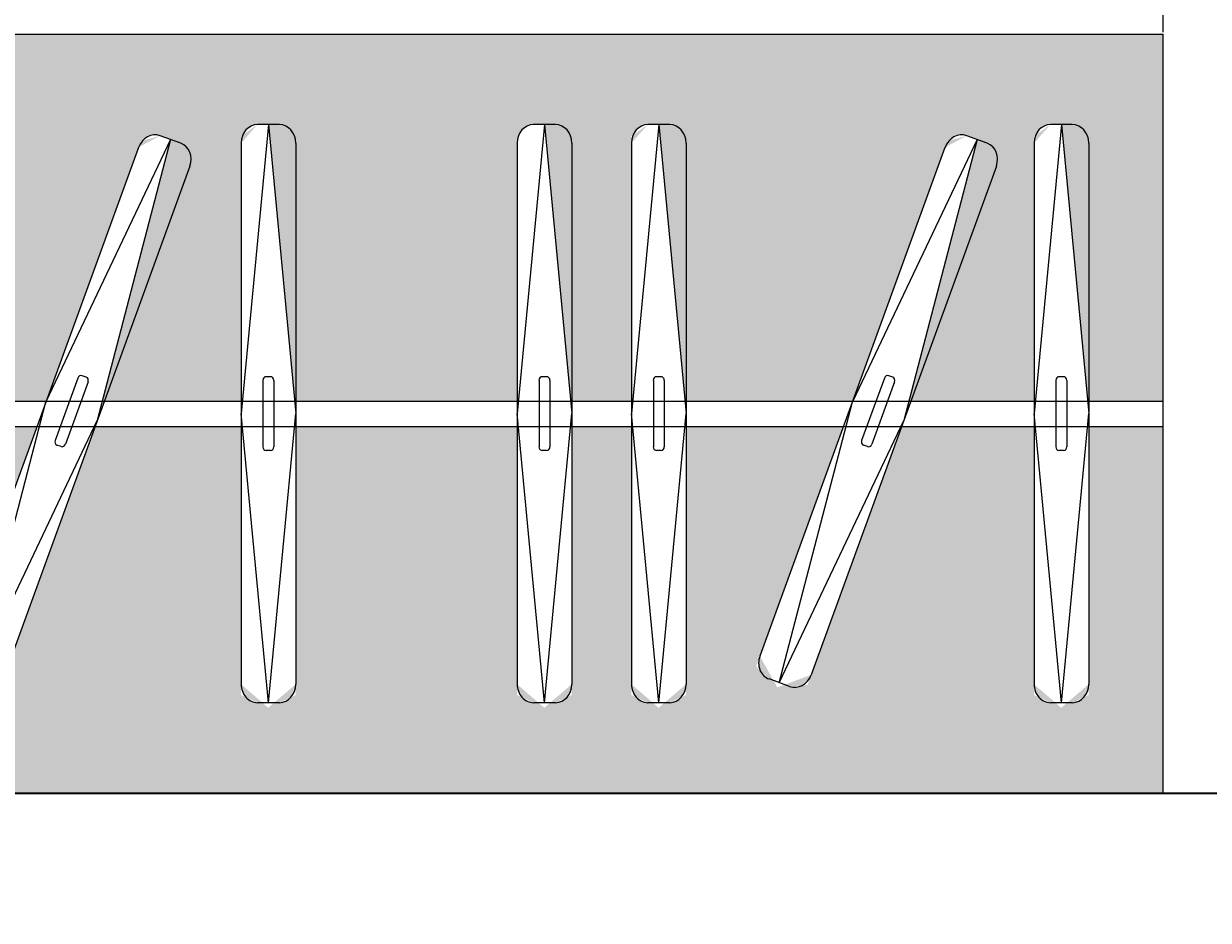
# Model space of a CAD drawing. Units: millimetres. Extents: x 27017497 to 27018854, y 7058029 to 7059154.
# Tile 40 of 91: x 27017655 to 27017689, y 7058433 to 7058459. Entities that reach past the tile are written whole.
import ezdxf

# ---------------------------------------------------------------- set-up
doc = ezdxf.new("R2010")
doc.units = ezdxf.units.MM
for name, color, linetype, lineweight in [('A-ANNO-DIMS', 2, 'Continuous', 18), ('A-FLOR-CASE', 8, 'Continuous', 20), ('A-FLOR-CASE-PATT', 44, 'Continuous', 13), ('A-WALL', 7, 'Continuous', 35)]:
    doc.layers.add(name, color=color, linetype=linetype, lineweight=lineweight)
doc.styles.get("Standard").update_dxf_attribs({"font": 'arial.ttf'})
doc.dimstyles.get("Standard").update_dxf_attribs({"dimtxt": 0.18, "dimasz": 0.18, "dimexe": 0.18, "dimexo": 0.0625, "dimgap": 0.09, "dimtad": 0, "dimtih": 1, "dimtoh": 1, "dimdec": 4, "dimzin": 0, "dimdsep": 46, "dimtxsty": 'Standard', "dimcen": 0.09, "dimadec": 0, "dimazin": 0, "dimtfac": 1, "dimtdec": 4, "dimtofl": 0, "dimtmove": 0, "dimatfit": 3, "dimfxl": 1, "dimtolj": 1, "dimtzin": 0, "dimarcsym": 0})

# ---------------------------------------------------------------- blocks, each defined once
blk = doc.blocks.new('WARDROBE-HANGING-WALL-BACKED')
for p, q in [((0, 21.737), (65.212, 21.737)), ((65.212, 0), (65.212, 21.737)), ((39.589, 19.152), (38.806, 10.877)), ((39.902, 19.152), (39.276, 19.152)), ((39.589, 19.152), (40.371, 10.877)), ((47.493, 19.152), (46.71, 10.877)), ((47.806, 19.152), (47.18, 19.152)), ((47.493, 19.152), (48.275, 10.877)), ((50.766, 19.152), (49.984, 10.877)), ((51.079, 19.152), (50.453, 19.152)), ((50.766, 19.152), (51.549, 10.877)), ((62.293, 19.152), (61.511, 10.877)), ((62.606, 19.152), (61.98, 19.152)), ((62.293, 19.152), (63.076, 10.877)), ((36.783, 18.725), (33.217, 11.217)), ((36.783, 18.725), (34.688, 10.682)), ((37.077, 18.618), (36.488, 18.833)), ((59.877, 18.725), (56.311, 11.217)), ((59.877, 18.725), (57.782, 10.682)), ((60.171, 18.618), (59.582, 18.833)), ((35.867, 18.497), (30.567, 3.937)), ((38.806, 18.624), (38.806, 3.13)), ((40.371, 18.624), (40.371, 3.13)), ((46.71, 18.624), (46.71, 3.13)), ((48.275, 18.624), (48.275, 3.13)), ((49.984, 18.624), (49.984, 3.13)), ((51.549, 18.624), (51.549, 3.13)), ((58.96, 18.497), (53.661, 3.937)), ((61.511, 18.624), (61.511, 3.13)), ((63.076, 18.624), (63.076, 3.13)), ((37.337, 17.961), (32.038, 3.402)), ((60.431, 17.961), (55.132, 3.402)), ((34.13, 11.896), (33.48, 10.109)), ((34.372, 11.92), (34.255, 11.963)), ((39.651, 11.933), (39.526, 11.933)), ((47.555, 11.933), (47.43, 11.933)), ((50.829, 11.933), (50.703, 11.933)), ((57.224, 11.896), (56.574, 10.109)), ((57.466, 11.92), (57.349, 11.963)), ((62.356, 11.933), (62.231, 11.933)), ((34.424, 11.789), (33.774, 10.002)), ((39.432, 11.828), (39.432, 9.926)), ((39.745, 11.828), (39.745, 9.926)), ((47.336, 11.828), (47.336, 9.926)), ((47.649, 11.828), (47.649, 9.926)), ((50.61, 11.828), (50.61, 9.926)), ((50.923, 11.828), (50.923, 9.926)), ((57.518, 11.789), (56.868, 10.002)), ((62.137, 11.828), (62.137, 9.926)), ((62.45, 11.828), (62.45, 9.926)), ((0, 11.231), (65.212, 11.231)), ((31.122, 3.173), (33.217, 11.217)), ((54.216, 3.173), (56.311, 11.217)), ((39.589, 2.602), (38.806, 10.877)), ((39.589, 2.602), (40.371, 10.877)), ((47.493, 2.602), (46.71, 10.877)), ((47.493, 2.602), (48.275, 10.877)), ((50.766, 2.602), (49.984, 10.877)), ((50.766, 2.602), (51.549, 10.877)), ((62.293, 2.602), (61.511, 10.877)), ((62.293, 2.602), (63.076, 10.877)), ((31.122, 3.173), (34.688, 10.682)), ((54.216, 3.173), (57.782, 10.682)), ((0, 10.506), (65.212, 10.506)), ((33.65, 9.935), (33.532, 9.978)), ((56.744, 9.935), (56.626, 9.978)), ((39.651, 9.821), (39.526, 9.821)), ((47.555, 9.821), (47.43, 9.821)), ((50.829, 9.821), (50.703, 9.821)), ((62.356, 9.821), (62.231, 9.821)), ((54.51, 3.066), (53.922, 3.28)), ((39.902, 2.602), (39.276, 2.602)), ((47.806, 2.602), (47.18, 2.602)), ((51.079, 2.602), (50.453, 2.602)), ((62.606, 2.602), (61.98, 2.602))]:
    blk.add_line(p, q)
for centre, major_axis, start_param, end_param in [((39.276, 18.624), (0, 0.528), 0, 1.570796), ((39.902, 18.624), (0, 0.528), 4.712389, 6.283185), ((47.18, 18.624), (0, 0.528), 0, 1.570796), ((47.806, 18.624), (0, 0.528), 4.712389, 6.283185), ((50.453, 18.624), (0, 0.528), 0, 1.570796), ((51.079, 18.624), (0, 0.528), 4.712389, 6.283185), ((61.98, 18.624), (0, 0.528), 0, 1.570796), ((62.606, 18.624), (0, 0.528), 4.712389, 6.283185), ((36.308, 18.336), (0.181, 0.496), 0, 1.570796), ((59.402, 18.336), (0.181, 0.496), 0, 1.570796), ((36.896, 18.122), (0.181, 0.496), -1.570796, 0), ((59.99, 18.122), (0.181, 0.496), -1.570796, 0), ((34.219, 11.864), (0.0361, 0.0993), 0, 1.570796), ((34.336, 11.821), (0.0361, 0.0993), 4.712389, 6.283185), ((39.526, 11.828), (0, 0.106), 0, 1.570796), ((39.651, 11.828), (0, 0.106), -1.570796, 0), ((47.43, 11.828), (0, 0.106), 0, 1.570796), ((47.555, 11.828), (0, 0.106), -1.570796, 0), ((50.703, 11.828), (0, 0.106), 0, 1.570796), ((50.829, 11.828), (0, 0.106), -1.570796, 0), ((57.313, 11.864), (0.0361, 0.0993), 0, 1.570796), ((57.43, 11.821), (0.0361, 0.0993), 4.712389, 6.283185), ((62.231, 11.828), (0, 0.106), 0, 1.570796), ((62.356, 11.828), (0, 0.106), -1.570796, 0), ((33.568, 10.077), (0.0361, 0.0993), 1.570796, 3.141593), ((33.686, 10.034), (0.0361, 0.0993), 3.141593, 4.712389), ((39.526, 9.926), (0, 0.106), 1.570796, 3.141593), ((39.651, 9.926), (0, 0.106), 3.141593, 4.712389), ((47.43, 9.926), (0, 0.106), 1.570796, 3.141593), ((47.555, 9.926), (0, 0.106), 3.141593, 4.712389), ((50.703, 9.926), (0, 0.106), 1.570796, 3.141593), ((50.829, 9.926), (0, 0.106), 3.141593, 4.712389), ((56.662, 10.077), (0.0361, 0.0993), 1.570796, 3.141593), ((56.78, 10.034), (0.0361, 0.0993), 3.141593, 4.712389), ((62.231, 9.926), (0, 0.106), 1.570796, 3.141593), ((62.356, 9.926), (0, 0.106), 3.141593, 4.712389), ((54.102, 3.776), (0.181, 0.496), 1.570796, 3.141593), ((54.691, 3.562), (0.181, 0.496), 3.141593, 4.712389), ((39.276, 3.13), (0, 0.528), 1.570796, 3.141593), ((39.902, 3.13), (0, 0.528), 3.141593, 4.712389), ((47.18, 3.13), (0, 0.528), 1.570796, 3.141593), ((47.806, 3.13), (0, 0.528), 3.141593, 4.712389), ((50.453, 3.13), (0, 0.528), 1.570796, 3.141593), ((51.079, 3.13), (0, 0.528), 3.141593, 4.712389), ((61.98, 3.13), (0, 0.528), 1.570796, 3.141593), ((62.606, 3.13), (0, 0.528), 3.141593, 4.712389)]:
    blk.add_ellipse(centre, major_axis=major_axis, ratio=0.888892, start_param=start_param, end_param=end_param)
blk = doc.blocks.new('*D45')
at = {"layer": 'A-ANNO-DIMS', "color": 0, "lineweight": -2, "transparency": 16777216}
for p, q in [((27017622.665, 7058458.704), (27017622.665, 7058468.604)), ((27017687.877, 7058458.704), (27017687.877, 7058468.604)), ((27017622.845, 7058468.424), (27017653.586, 7058468.424)), ((27017687.697, 7058468.424), (27017656.955, 7058468.424))]:
    blk.add_line(p, q, dxfattribs=at)
at = {"layer": 'A-ANNO-DIMS', "color": 0, "transparency": 16777216}
for points in [[(27017622.845, 7058468.454), (27017622.845, 7058468.394), (27017622.665, 7058468.424)], [(27017687.697, 7058468.454), (27017687.697, 7058468.394), (27017687.877, 7058468.424)]]:
    blk.add_solid(points, dxfattribs=at)
at = {"layer": 'Defpoints', "color": 0, "transparency": 16777216}
for p in [(27017687.877, 7058468.424), (27017622.665, 7058458.642), (27017687.877, 7058458.642)]:
    blk.add_point(p, dxfattribs=at)
at = {"layer": 'A-ANNO-DIMS', "color": 0, "transparency": 16777216, "insert": (27017655.271, 7058468.424), "char_height": 0.18, "attachment_point": 5}
blk.add_mtext('\\A1;WALL WARDROBE 65 TYP.', dxfattribs=at)
blk = doc.blocks.new('*D48')
at = {"layer": 'A-ANNO-DIMS', "color": 0, "lineweight": -2, "transparency": 16777216}
for p, q in [((27018463.498, 7058622.912), (27017497.536, 7058622.912)), ((27017497.716, 7058622.732), (27017497.716, 7058357.753)), ((27017497.716, 7058092.41), (27017497.716, 7058357.389)), ((27018555.129, 7058092.23), (27017497.536, 7058092.23))]:
    blk.add_line(p, q, dxfattribs=at)
at = {"layer": 'A-ANNO-DIMS', "color": 0, "transparency": 16777216}
for points in [[(27017497.686, 7058622.732), (27017497.746, 7058622.732), (27017497.716, 7058622.912)], [(27017497.686, 7058092.41), (27017497.746, 7058092.41), (27017497.716, 7058092.23)]]:
    blk.add_solid(points, dxfattribs=at)
at = {"layer": 'Defpoints', "color": 0, "transparency": 16777216}
for p in [(27018463.561, 7058622.912), (27017497.716, 7058092.23), (27018555.192, 7058092.23)]:
    blk.add_point(p, dxfattribs=at)
at = {"layer": 'A-ANNO-DIMS', "color": 0, "transparency": 16777216, "insert": (27017497.716, 7058357.571), "char_height": 0.18, "attachment_point": 5}
blk.add_mtext('\\A1;530.7', dxfattribs=at)

msp = doc.modelspace()

# ---------------------------------------------------------------- hatches: boundary and pattern name
at = {"layer": 'A-FLOR-CASE-PATT'}
h = msp.add_hatch(color=256, dxfattribs=at)
h.dxf.hatch_style = 1
edge = h.paths.add_edge_path()
edge.add_line((27017641.545, 7058447.411), (27017637.752, 7058447.411))
edge.add_line((27017637.752, 7058447.411), (27017635.06, 7058440.016))
edge.add_ellipse((27017634.725, 7058440.467), major_axis=(0.181, 0.496), ratio=0.888892, start_angle=180, end_angle=270, ccw=False)
edge.add_line((27017634.184, 7058439.939), (27017634.19, 7058439.951))
edge.add_ellipse((27017634.137, 7058440.681), major_axis=(0.181, 0.496), ratio=0.888892, start_angle=90, end_angle=180, ccw=False)
edge.add_line((27017633.59, 7058440.551), (27017636.086, 7058447.411))
edge.add_line((27017636.086, 7058447.411), (27017631.583, 7058447.411))
edge.add_line((27017631.583, 7058447.411), (27017631.583, 7058439.726))
edge.add_ellipse((27017631.113, 7058440.035), major_axis=(0, 0.528), ratio=0.888892, start_angle=180, end_angle=270, ccw=False)
edge.add_line((27017630.786, 7058439.354), (27017630.787, 7058439.367))
edge.add_ellipse((27017630.487, 7058440.035), major_axis=(0, 0.528), ratio=0.888892, start_angle=90, end_angle=180, ccw=False)
edge.add_line((27017630.018, 7058439.726), (27017630.018, 7058447.411))
edge.add_line((27017630.018, 7058447.411), (27017628.31, 7058447.411))
edge.add_line((27017628.31, 7058447.411), (27017628.31, 7058439.726))
edge.add_ellipse((27017627.84, 7058440.035), major_axis=(0, 0.528), ratio=0.888892, start_angle=180, end_angle=270, ccw=False)
edge.add_line((27017627.513, 7058439.354), (27017627.514, 7058439.367))
edge.add_ellipse((27017627.214, 7058440.035), major_axis=(0, 0.528), ratio=0.888892, start_angle=90, end_angle=180, ccw=False)
edge.add_line((27017626.745, 7058439.726), (27017626.745, 7058447.411))
edge.add_line((27017626.745, 7058447.411), (27017622.666, 7058447.411))
edge.add_line((27017622.666, 7058447.411), (27017622.666, 7058436.912))
edge.add_line((27017622.666, 7058436.912), (27017687.877, 7058436.912))
edge.add_line((27017687.877, 7058436.912), (27017687.877, 7058447.411))
edge.add_line((27017687.877, 7058447.411), (27017685.741, 7058447.411))
edge.add_line((27017685.741, 7058447.411), (27017685.741, 7058439.726))
edge.add_ellipse((27017685.271, 7058440.035), major_axis=(0, 0.528), ratio=0.888892, start_angle=180, end_angle=270, ccw=False)
edge.add_line((27017684.944, 7058439.354), (27017684.945, 7058439.367))
edge.add_ellipse((27017684.645, 7058440.035), major_axis=(0, 0.528), ratio=0.888892, start_angle=90, end_angle=180, ccw=False)
edge.add_line((27017684.176, 7058439.726), (27017684.176, 7058447.411))
edge.add_line((27017684.176, 7058447.411), (27017680.383, 7058447.411))
edge.add_line((27017680.383, 7058447.411), (27017677.691, 7058440.016))
edge.add_ellipse((27017677.356, 7058440.467), major_axis=(0.181, 0.496), ratio=0.888892, start_angle=180, end_angle=270, ccw=False)
edge.add_line((27017676.815, 7058439.939), (27017676.821, 7058439.951))
edge.add_ellipse((27017676.767, 7058440.681), major_axis=(0.181, 0.496), ratio=0.888892, start_angle=90, end_angle=180, ccw=False)
edge.add_line((27017676.22, 7058440.551), (27017678.717, 7058447.411))
edge.add_line((27017678.717, 7058447.411), (27017674.214, 7058447.411))
edge.add_line((27017674.214, 7058447.411), (27017674.214, 7058439.726))
edge.add_ellipse((27017673.744, 7058440.035), major_axis=(0, 0.528), ratio=0.888892, start_angle=180, end_angle=270, ccw=False)
edge.add_line((27017673.417, 7058439.354), (27017673.418, 7058439.367))
edge.add_ellipse((27017673.118, 7058440.035), major_axis=(0, 0.528), ratio=0.888892, start_angle=90, end_angle=180, ccw=False)
edge.add_line((27017672.649, 7058439.726), (27017672.649, 7058447.411))
edge.add_line((27017672.649, 7058447.411), (27017670.94, 7058447.411))
edge.add_line((27017670.94, 7058447.411), (27017670.94, 7058439.726))
edge.add_ellipse((27017670.471, 7058440.035), major_axis=(0, 0.528), ratio=0.888892, start_angle=180, end_angle=270, ccw=False)
edge.add_line((27017670.143, 7058439.354), (27017670.145, 7058439.367))
edge.add_ellipse((27017669.845, 7058440.035), major_axis=(0, 0.528), ratio=0.888892, start_angle=90, end_angle=180, ccw=False)
edge.add_line((27017669.375, 7058439.726), (27017669.375, 7058447.411))
edge.add_line((27017669.375, 7058447.411), (27017663.036, 7058447.411))
edge.add_line((27017663.036, 7058447.411), (27017663.036, 7058439.726))
edge.add_ellipse((27017662.567, 7058440.035), major_axis=(0, 0.528), ratio=0.888892, start_angle=180, end_angle=270, ccw=False)
edge.add_line((27017662.239, 7058439.354), (27017662.241, 7058439.367))
edge.add_ellipse((27017661.941, 7058440.035), major_axis=(0, 0.528), ratio=0.888892, start_angle=90, end_angle=180, ccw=False)
edge.add_line((27017661.471, 7058439.726), (27017661.471, 7058447.411))
edge.add_line((27017661.471, 7058447.411), (27017657.289, 7058447.411))
edge.add_line((27017657.289, 7058447.411), (27017654.597, 7058440.016))
edge.add_ellipse((27017654.262, 7058440.467), major_axis=(0.181, 0.496), ratio=0.888892, start_angle=180, end_angle=270, ccw=False)
edge.add_line((27017653.721, 7058439.939), (27017653.727, 7058439.951))
edge.add_ellipse((27017653.673, 7058440.681), major_axis=(0.181, 0.496), ratio=0.888892, start_angle=90, end_angle=180, ccw=False)
edge.add_line((27017653.126, 7058440.551), (27017655.623, 7058447.411))
edge.add_line((27017655.623, 7058447.411), (27017652.621, 7058447.411))
edge.add_line((27017652.621, 7058447.411), (27017652.621, 7058439.726))
edge.add_ellipse((27017652.151, 7058440.035), major_axis=(0, 0.528), ratio=0.888892, start_angle=180, end_angle=270, ccw=False)
edge.add_line((27017651.824, 7058439.354), (27017651.825, 7058439.367))
edge.add_ellipse((27017651.525, 7058440.035), major_axis=(0, 0.528), ratio=0.888892, start_angle=90, end_angle=180, ccw=False)
edge.add_line((27017651.056, 7058439.726), (27017651.056, 7058447.411))
edge.add_line((27017651.056, 7058447.411), (27017649.348, 7058447.411))
edge.add_line((27017649.348, 7058447.411), (27017649.348, 7058439.726))
edge.add_ellipse((27017648.878, 7058440.035), major_axis=(0, 0.528), ratio=0.888892, start_angle=180, end_angle=270, ccw=False)
edge.add_line((27017648.551, 7058439.354), (27017648.552, 7058439.367))
edge.add_ellipse((27017648.252, 7058440.035), major_axis=(0, 0.528), ratio=0.888892, start_angle=90, end_angle=180, ccw=False)
edge.add_line((27017647.783, 7058439.726), (27017647.783, 7058447.411))
edge.add_line((27017647.783, 7058447.411), (27017643.11, 7058447.411))
edge.add_line((27017643.11, 7058447.411), (27017643.11, 7058439.726))
edge.add_ellipse((27017642.641, 7058440.035), major_axis=(0, 0.528), ratio=0.888892, start_angle=180, end_angle=270, ccw=False)
edge.add_line((27017642.313, 7058439.354), (27017642.314, 7058439.367))
edge.add_ellipse((27017642.015, 7058440.035), major_axis=(0, 0.528), ratio=0.888892, start_angle=90, end_angle=180, ccw=False)
edge.add_line((27017641.545, 7058439.726), (27017641.545, 7058447.411))
edge = h.paths.add_edge_path()
edge.add_line((27017669.845, 7058456.057), (27017670.158, 7058456.057))
edge.add_line((27017670.158, 7058456.057), (27017670.907, 7058448.136))
edge.add_line((27017670.907, 7058448.136), (27017672.649, 7058448.136))
edge.add_line((27017672.649, 7058448.136), (27017672.649, 7058455.723))
edge.add_ellipse((27017673.118, 7058455.529), major_axis=(0, 0.528), ratio=0.888892, start_angle=0, end_angle=90, ccw=False)
edge.add_line((27017673.118, 7058456.057), (27017673.431, 7058456.057))
edge.add_line((27017673.431, 7058456.057), (27017674.18, 7058448.136))
edge.add_line((27017674.18, 7058448.136), (27017678.981, 7058448.136))
edge.add_line((27017678.981, 7058448.136), (27017681.692, 7058455.583))
edge.add_ellipse((27017682.067, 7058455.241), major_axis=(0.181, 0.496), ratio=0.888892, start_angle=0, end_angle=90, ccw=False)
edge.add_line((27017682.247, 7058455.738), (27017682.542, 7058455.63))
edge.add_line((27017682.542, 7058455.63), (27017680.59, 7058448.136))
edge.add_line((27017680.59, 7058448.136), (27017684.176, 7058448.136))
edge.add_line((27017684.176, 7058448.136), (27017684.176, 7058455.723))
edge.add_ellipse((27017684.645, 7058455.529), major_axis=(0, 0.528), ratio=0.888892, start_angle=0, end_angle=90, ccw=False)
edge.add_line((27017684.645, 7058456.057), (27017684.958, 7058456.057))
edge.add_line((27017684.958, 7058456.057), (27017685.707, 7058448.136))
edge.add_line((27017685.707, 7058448.136), (27017687.877, 7058448.136))
edge.add_line((27017687.877, 7058448.136), (27017687.877, 7058458.642))
edge.add_line((27017687.877, 7058458.642), (27017622.666, 7058458.642))
edge.add_line((27017622.666, 7058458.642), (27017622.666, 7058448.136))
edge.add_line((27017622.666, 7058448.136), (27017626.745, 7058448.136))
edge.add_line((27017626.745, 7058448.136), (27017626.745, 7058455.723))
edge.add_ellipse((27017627.214, 7058455.529), major_axis=(0, 0.528), ratio=0.888892, start_angle=0, end_angle=90, ccw=False)
edge.add_line((27017627.214, 7058456.057), (27017627.527, 7058456.057))
edge.add_line((27017627.527, 7058456.057), (27017628.276, 7058448.136))
edge.add_line((27017628.276, 7058448.136), (27017630.018, 7058448.136))
edge.add_line((27017630.018, 7058448.136), (27017630.018, 7058455.723))
edge.add_ellipse((27017630.487, 7058455.529), major_axis=(0, 0.528), ratio=0.888892, start_angle=0, end_angle=90, ccw=False)
edge.add_line((27017630.487, 7058456.057), (27017630.8, 7058456.057))
edge.add_line((27017630.8, 7058456.057), (27017631.549, 7058448.136))
edge.add_line((27017631.549, 7058448.136), (27017636.35, 7058448.136))
edge.add_line((27017636.35, 7058448.136), (27017639.061, 7058455.583))
edge.add_ellipse((27017639.436, 7058455.241), major_axis=(0.181, 0.496), ratio=0.888892, start_angle=0, end_angle=90, ccw=False)
edge.add_line((27017639.617, 7058455.738), (27017639.911, 7058455.63))
edge.add_line((27017639.911, 7058455.63), (27017637.959, 7058448.136))
edge.add_line((27017637.959, 7058448.136), (27017641.545, 7058448.136))
edge.add_line((27017641.545, 7058448.136), (27017641.545, 7058455.723))
edge.add_ellipse((27017642.015, 7058455.529), major_axis=(0, 0.528), ratio=0.888892, start_angle=0, end_angle=90, ccw=False)
edge.add_line((27017642.015, 7058456.057), (27017642.328, 7058456.057))
edge.add_line((27017642.328, 7058456.057), (27017643.077, 7058448.136))
edge.add_line((27017643.077, 7058448.136), (27017647.783, 7058448.136))
edge.add_line((27017647.783, 7058448.136), (27017647.783, 7058455.723))
edge.add_ellipse((27017648.252, 7058455.529), major_axis=(0, 0.528), ratio=0.888892, start_angle=0, end_angle=90, ccw=False)
edge.add_line((27017648.252, 7058456.057), (27017648.565, 7058456.057))
edge.add_line((27017648.565, 7058456.057), (27017649.314, 7058448.136))
edge.add_line((27017649.314, 7058448.136), (27017651.056, 7058448.136))
edge.add_line((27017651.056, 7058448.136), (27017651.056, 7058455.723))
edge.add_ellipse((27017651.525, 7058455.529), major_axis=(0, 0.528), ratio=0.888892, start_angle=0, end_angle=90, ccw=False)
edge.add_line((27017651.525, 7058456.057), (27017651.838, 7058456.057))
edge.add_line((27017651.838, 7058456.057), (27017652.587, 7058448.136))
edge.add_line((27017652.587, 7058448.136), (27017655.887, 7058448.136))
edge.add_line((27017655.887, 7058448.136), (27017658.598, 7058455.583))
edge.add_ellipse((27017658.973, 7058455.241), major_axis=(0.181, 0.496), ratio=0.888892, start_angle=0, end_angle=90, ccw=False)
edge.add_line((27017659.153, 7058455.738), (27017659.448, 7058455.63))
edge.add_line((27017659.448, 7058455.63), (27017657.496, 7058448.136))
edge.add_line((27017657.496, 7058448.136), (27017661.471, 7058448.136))
edge.add_line((27017661.471, 7058448.136), (27017661.471, 7058455.723))
edge.add_ellipse((27017661.941, 7058455.529), major_axis=(0, 0.528), ratio=0.888892, start_angle=0, end_angle=90, ccw=False)
edge.add_line((27017661.941, 7058456.057), (27017662.254, 7058456.057))
edge.add_line((27017662.254, 7058456.057), (27017663.003, 7058448.136))
edge.add_line((27017663.003, 7058448.136), (27017669.375, 7058448.136))
edge.add_line((27017669.375, 7058448.136), (27017669.375, 7058455.723))
edge.add_ellipse((27017669.845, 7058455.529), major_axis=(0, 0.528), ratio=0.888892, start_angle=0, end_angle=90, ccw=False)

# ---------------------------------------------------------------- linework, layer by layer
at = {"layer": 'A-WALL'}
msp.add_line((27017622.666, 7058436.912), (27017716.811, 7058436.912), dxfattribs=at)

# ---------------------------------------------------------------- block references
at = {"layer": 'A-FLOR-CASE'}
msp.add_blockref('WARDROBE-HANGING-WALL-BACKED', (27017622.665, 7058436.905), dxfattribs=at)

# ---------------------------------------------------------------- dimensions: what is measured, and where the dimension line sits
at = {"layer": 'A-ANNO-DIMS'}
dim = msp.add_linear_dim(base=(27017497.716, 7058092.23), p1=(27018463.561, 7058622.912), p2=(27018555.192, 7058092.23), angle=90, dimstyle='Standard', override={"dimdec": 1, "dimlfac": 1, "dimrnd": 0, "dimzin": 0, "dimdsep": 46, "dimlunit": 2}, dxfattribs=at)
dim.commit()
dim.dimension.update_dxf_attribs({"geometry": '*D48', "text_midpoint": (27017497.716, 7058357.571)})
dim = msp.add_linear_dim(base=(27017687.877, 7058468.424), p1=(27017622.665, 7058458.642), p2=(27017687.877, 7058458.642), text='WALL WARDROBE <> TYP.', dimstyle='Standard', override={"dimdec": 0, "dimlfac": 1, "dimrnd": 0, "dimzin": 0, "dimdsep": 46, "dimlunit": 2}, dxfattribs=at)
dim.commit()
dim.dimension.update_dxf_attribs({"geometry": '*D45', "text_midpoint": (27017655.271, 7058468.424)})

doc.saveas('drawing.dxf')
